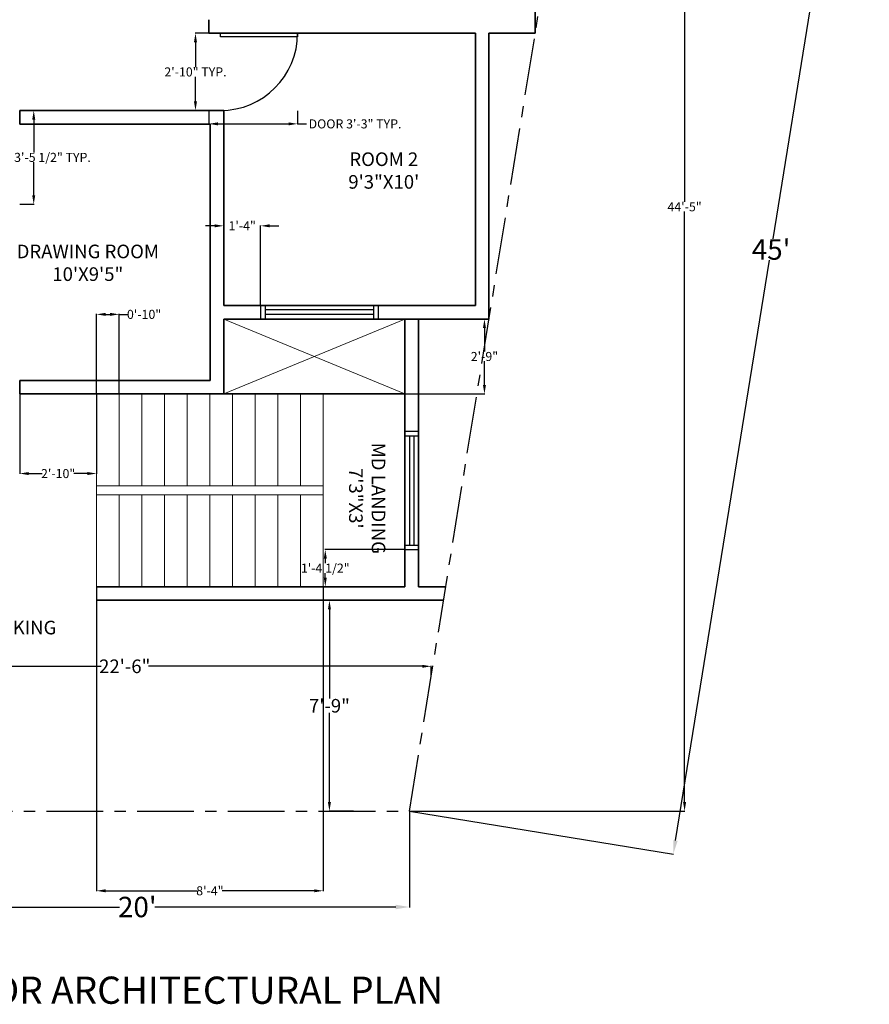
# Model space of a CAD drawing. Units: inches. Extents: x 1778 to 2384, y 384 to 1080.
# Tile 2 of 3: x 2009 to 2384, y 406 to 841. Entities that reach past the tile are written whole.
import ezdxf

# ---------------------------------------------------------------- set-up
doc = ezdxf.new("R2010")
doc.units = ezdxf.units.IN
doc.header["$MEASUREMENT"] = 0
doc.linetypes.add('CENTER', pattern=[2, 1.25, -0.25, 0.25, -0.25])
for name, color, linetype, lineweight in [('A-ANNO-DIMS', 2, 'Continuous', 18), ('A-ANNO-TEXT', 72, 'Continuous', 25), ('A-AREA-IDEN', 1, 'Continuous', 18), ('A-FLOR-STRS', 7, 'Continuous', 18), ('A-GLAZ', 4, 'Continuous', 18), ('A-WALL', 7, 'Continuous', 35), ('C-PROP', 13, 'CENTER', 25), ('DOOR', 13, 'Continuous', 25)]:
    doc.layers.add(name, color=color, linetype=linetype, lineweight=lineweight)
doc.styles.get("Standard").update_dxf_attribs({"font": 'arial.ttf'})
doc.dimstyles.get("Standard").update_dxf_attribs({"dimtxt": 4, "dimasz": 4, "dimexe": 0.18, "dimexo": 0.0625, "dimgap": 0.09, "dimtad": 0, "dimtih": 1, "dimtoh": 1, "dimdec": 0, "dimzin": 0, "dimdsep": 46, "dimlunit": 3, "dimtxsty": 'Standard', "dimcen": 0.09, "dimadec": 0, "dimazin": 0, "dimtfac": 1, "dimtdec": 0, "dimtofl": 0, "dimtmove": 0, "dimatfit": 3, "dimfxl": 1, "dimtolj": 1, "dimtzin": 0, "dimarcsym": 0})

# ---------------------------------------------------------------- blocks, each defined once
blk = doc.blocks.new('*D1')
at = {"layer": 'A-ANNO-DIMS', "color": 0, "lineweight": -2, "transparency": 16777216}
for p, q in [((2267.72, 1024.58), (2384.25, 1005.72)), ((2383.11, 999.82), (2341.67, 743.88)), ((2298.72, 478.61), (2340.16, 734.55)), ((2181.42, 491.52), (2297.94, 472.66))]:
    blk.add_line(p, q, dxfattribs=at)
at = {"layer": 'A-ANNO-DIMS', "color": 0, "transparency": 16777216}
for points in [[(2382.12, 999.98), (2384.1, 999.66), (2384.07, 1005.75)], [(2297.74, 478.77), (2299.71, 478.45), (2297.77, 472.69)]]:
    blk.add_solid(points, dxfattribs=at)
at = {"layer": 'Defpoints', "color": 0, "transparency": 16777216}
for p in [(2267.66, 1024.59), (2384.07, 1005.75), (2181.36, 491.53)]:
    blk.add_point(p, dxfattribs=at)
at = {"layer": 'A-ANNO-DIMS', "color": 0, "transparency": 16777216, "insert": (2340.92, 739.22), "char_height": 9, "attachment_point": 5}
blk.add_mtext("\\A1;45'", dxfattribs=at)
blk = doc.blocks.new('*D2')
at = {"layer": 'A-ANNO-DIMS', "color": 0, "lineweight": -2, "transparency": 16777216}
for p, q in [((1941.36, 491.47), (1941.36, 449.11)), ((2181.36, 491.47), (2181.36, 449.11)), ((1947.36, 449.29), (2053.55, 449.29)), ((2175.36, 449.29), (2069.16, 449.29))]:
    blk.add_line(p, q, dxfattribs=at)
at = {"layer": 'A-ANNO-DIMS', "color": 0, "transparency": 16777216}
for points in [[(1947.36, 450.29), (1947.36, 448.29), (1941.36, 449.29)], [(2175.36, 450.29), (2175.36, 448.29), (2181.36, 449.29)]]:
    blk.add_solid(points, dxfattribs=at)
at = {"layer": 'Defpoints', "color": 0, "transparency": 16777216}
for p in [(1941.36, 491.53), (2181.36, 491.53), (2181.36, 449.29)]:
    blk.add_point(p, dxfattribs=at)
at = {"layer": 'A-ANNO-DIMS', "color": 0, "transparency": 16777216, "insert": (2061.36, 449.29), "char_height": 9, "attachment_point": 5}
blk.add_mtext("\\A1;20'", dxfattribs=at)
blk = doc.blocks.new('*D4')
at = {"layer": 'A-ANNO-DIMS', "color": 0, "lineweight": -2, "transparency": 16777216}
for p, q in [((2238.23, 1077.18), (2031.58, 987.25)), ((2267.63, 1024.65), (2243.66, 1079.74)), ((1809.1, 890.44), (2015.76, 980.36)), ((1827.5, 833.12), (1803.53, 888.21))]:
    blk.add_line(p, q, dxfattribs=at)
at = {"layer": 'A-ANNO-DIMS', "color": 0, "transparency": 16777216}
for points in [[(2237.83, 1078.09), (2238.63, 1076.26), (2243.73, 1079.57)], [(1808.7, 891.35), (1809.5, 889.52), (1803.6, 888.04)]]:
    blk.add_solid(points, dxfattribs=at)
at = {"layer": 'Defpoints', "color": 0, "transparency": 16777216}
for p in [(2243.73, 1079.57), (2267.66, 1024.59), (1827.53, 833.06)]:
    blk.add_point(p, dxfattribs=at)
at = {"layer": 'A-ANNO-DIMS', "color": 0, "transparency": 16777216, "insert": (2023.67, 983.81), "char_height": 9, "attachment_point": 5}
blk.add_mtext("\\A1;40'", dxfattribs=at)
blk = doc.blocks.new('*D9')
at = {"layer": 'A-ANNO-DIMS', "color": 0, "lineweight": -2, "transparency": 16777216}
for p, q in [((1920.61, 553.84), (1920.61, 555.61)), ((1924.61, 555.43), (2045.38, 555.43)), ((2187.04, 555.43), (2066.27, 555.43)), ((2191.04, 551.41), (2191.04, 555.61))]:
    blk.add_line(p, q, dxfattribs=at)
at = {"layer": 'A-ANNO-DIMS', "color": 0, "transparency": 16777216}
for points in [[(1924.61, 556.1), (1924.61, 554.77), (1920.61, 555.43)], [(2187.04, 556.1), (2187.04, 554.77), (2191.04, 555.43)]]:
    blk.add_solid(points, dxfattribs=at)
at = {"layer": 'Defpoints', "color": 0, "transparency": 16777216}
for p in [(1920.61, 555.43), (1920.61, 553.77), (2191.04, 551.35)]:
    blk.add_point(p, dxfattribs=at)
at = {"layer": 'A-ANNO-DIMS', "color": 0, "transparency": 16777216, "insert": (2055.83, 555.43), "char_height": 6, "attachment_point": 5}
blk.add_mtext('\\A1;22\'-6"', dxfattribs=at)
blk = doc.blocks.new('*D12')
at = {"layer": 'A-ANNO-DIMS', "color": 0, "lineweight": -2, "transparency": 16777216}
for p, q in [((2156.73, 584.53), (2145.93, 584.53)), ((2146.11, 580.53), (2146.11, 541.19)), ((2146.11, 495.53), (2146.11, 534.88)), ((2156.73, 491.53), (2145.93, 491.53))]:
    blk.add_line(p, q, dxfattribs=at)
at = {"layer": 'A-ANNO-DIMS', "color": 0, "transparency": 16777216}
for points in [[(2145.44, 580.53), (2146.77, 580.53), (2146.11, 584.53)], [(2145.44, 495.53), (2146.77, 495.53), (2146.11, 491.53)]]:
    blk.add_solid(points, dxfattribs=at)
at = {"layer": 'Defpoints', "color": 0, "transparency": 16777216}
for p in [(2146.11, 584.53), (2156.8, 584.53), (2156.8, 491.53)]:
    blk.add_point(p, dxfattribs=at)
at = {"layer": 'A-ANNO-DIMS', "color": 0, "transparency": 16777216, "insert": (2146.11, 538.03), "char_height": 6, "attachment_point": 5}
blk.add_mtext('\\A1;7\'-9"', dxfattribs=at)
blk = doc.blocks.new('*U14')
for p, q in [((0, 0), (0, -6)), ((40, 0), (40, -6))]:
    blk.add_line(p, q)
blk.add_lwpolyline([(0, 0), (0, 40), (1.75, 40), (1.75, 0)], close=True)
blk.add_arc((0, 0), 40, 0, 90)
blk = doc.blocks.new('DOOR')
blk.add_blockref('*U14', (1810.9, 983.44))
blk = doc.blocks.new('WINDOW')
for p, q in [((1664.47, 998.33), (1658.47, 998.33)), ((1658.47, 950.33), (1664.47, 950.33))]:
    blk.add_line(p, q)
at = {"layer": 'DOOR'}
for p, q in [((1664.47, 1000.33), (1658.47, 1000.33)), ((1660.47, 998.33), (1660.47, 950.33)), ((1662.47, 998.33), (1662.47, 950.33)), ((1658.47, 948.33), (1664.47, 948.33))]:
    blk.add_line(p, q, dxfattribs=at)
blk = doc.blocks.new('WIN')
at = {"layer": 'Defpoints'}
for p, q in [((1658.47, 1000.33), (1658.47, 948.33)), ((1664.47, 1000.33), (1664.47, 948.33))]:
    blk.add_line(p, q, dxfattribs=at)
at = {"layer": 'DOOR'}
blk.add_blockref('WINDOW', (0, 0), dxfattribs=at)
blk = doc.blocks.new('*D21')
at = {"layer": 'A-ANNO-DIMS', "color": 0, "lineweight": -2, "transparency": 16777216}
for p, q in [((2009.54, 800.53), (2015.86, 800.53)), ((2015.68, 796.53), (2015.68, 782.01)), ((2015.68, 763.16), (2015.68, 777.68)), ((2009.54, 759.16), (2015.86, 759.16))]:
    blk.add_line(p, q, dxfattribs=at)
at = {"layer": 'A-ANNO-DIMS', "color": 0, "transparency": 16777216}
for points in [[(2015.01, 796.53), (2016.35, 796.53), (2015.68, 800.53)], [(2015.01, 763.16), (2016.35, 763.16), (2015.68, 759.16)]]:
    blk.add_solid(points, dxfattribs=at)
at = {"layer": 'Defpoints', "color": 0, "transparency": 16777216}
for p in [(2009.47, 800.53), (2009.47, 759.16), (2015.68, 759.16)]:
    blk.add_point(p, dxfattribs=at)
at = {"layer": 'A-ANNO-DIMS', "color": 0, "transparency": 16777216, "insert": (2015.68, 779.85), "char_height": 4, "attachment_point": 5}
blk.add_mtext('\\A1;DOOR 3\'-5 1/2" TYP.', dxfattribs=at)
blk = doc.blocks.new('*D23')
at = {"layer": 'A-ANNO-DIMS', "color": 0, "lineweight": -2, "transparency": 16777216}
for p, q in [((2092.89, 800.45), (2092.89, 794.45)), ((2132.06, 800.45), (2132.06, 794.45)), ((2096.89, 794.63), (2128.06, 794.63)), ((2132.06, 794.63), (2136.06, 794.63))]:
    blk.add_line(p, q, dxfattribs=at)
at = {"layer": 'A-ANNO-DIMS', "color": 0, "transparency": 16777216}
for points in [[(2096.89, 795.3), (2096.89, 793.97), (2092.89, 794.63)], [(2128.06, 795.3), (2128.06, 793.97), (2132.06, 794.63)]]:
    blk.add_solid(points, dxfattribs=at)
at = {"layer": 'Defpoints', "color": 0, "transparency": 16777216}
for p in [(2092.89, 800.51), (2132.06, 800.51), (2132.06, 794.63)]:
    blk.add_point(p, dxfattribs=at)
at = {"layer": 'A-ANNO-DIMS', "color": 0, "transparency": 16777216, "insert": (2157.4, 794.63), "char_height": 4, "attachment_point": 5}
blk.add_mtext('\\A1;DOOR 3\'-3" TYP.', dxfattribs=at)
blk = doc.blocks.new('*D24')
at = {"layer": 'A-ANNO-DIMS', "color": 0, "lineweight": -2, "transparency": 16777216}
for p, q in [((2092.83, 834.57), (2086.84, 834.57)), ((2087.02, 830.57), (2087.02, 819.67)), ((2087.02, 804.51), (2087.02, 815.41)), ((2092.83, 800.51), (2086.84, 800.51))]:
    blk.add_line(p, q, dxfattribs=at)
at = {"layer": 'A-ANNO-DIMS', "color": 0, "transparency": 16777216}
for points in [[(2086.35, 830.57), (2087.69, 830.57), (2087.02, 834.57)], [(2086.35, 804.51), (2087.69, 804.51), (2087.02, 800.51)]]:
    blk.add_solid(points, dxfattribs=at)
at = {"layer": 'Defpoints', "color": 0, "transparency": 16777216}
for p in [(2092.89, 834.57), (2087.02, 800.51), (2092.89, 800.51)]:
    blk.add_point(p, dxfattribs=at)
at = {"layer": 'A-ANNO-DIMS', "color": 0, "transparency": 16777216, "insert": (2087.02, 817.54), "char_height": 4, "attachment_point": 5}
blk.add_mtext('\\A1;2\'-10" TYP.', dxfattribs=at)
blk = doc.blocks.new('*D35')
at = {"layer": 'A-ANNO-DIMS', "color": 0, "lineweight": -2, "transparency": 16777216}
for p, q in [((2267.72, 1024.59), (2302.94, 1024.59)), ((2302.76, 1020.59), (2302.76, 760.19)), ((2302.76, 495.53), (2302.76, 755.94)), ((2181.42, 491.53), (2302.94, 491.53))]:
    blk.add_line(p, q, dxfattribs=at)
at = {"layer": 'A-ANNO-DIMS', "color": 0, "transparency": 16777216}
for points in [[(2302.09, 1020.59), (2303.43, 1020.59), (2302.76, 1024.59)], [(2302.09, 495.53), (2303.43, 495.53), (2302.76, 491.53)]]:
    blk.add_solid(points, dxfattribs=at)
at = {"layer": 'Defpoints', "color": 0, "transparency": 16777216}
for p in [(2267.66, 1024.59), (2302.76, 1024.59), (2181.36, 491.53)]:
    blk.add_point(p, dxfattribs=at)
at = {"layer": 'A-ANNO-DIMS', "color": 0, "transparency": 16777216, "insert": (2302.76, 758.06), "char_height": 4, "attachment_point": 5}
blk.add_mtext('\\A1;44\'-5"', dxfattribs=at)
blk = doc.blocks.new('*D36')
at = {"layer": 'A-ANNO-DIMS', "color": 0, "lineweight": -2, "transparency": 16777216}
for p, q in [((1827.53, 833.13), (1827.53, 1059.87)), ((1831.53, 1059.69), (2040.63, 1059.69)), ((2263.66, 1059.69), (2054.55, 1059.69)), ((2267.66, 1024.66), (2267.66, 1059.87))]:
    blk.add_line(p, q, dxfattribs=at)
at = {"layer": 'A-ANNO-DIMS', "color": 0, "transparency": 16777216}
for points in [[(1831.53, 1060.36), (1831.53, 1059.03), (1827.53, 1059.69)], [(2263.66, 1060.36), (2263.66, 1059.03), (2267.66, 1059.69)]]:
    blk.add_solid(points, dxfattribs=at)
at = {"layer": 'Defpoints', "color": 0, "transparency": 16777216}
for p in [(2267.66, 1059.69), (2267.66, 1024.59), (1827.53, 833.06)]:
    blk.add_point(p, dxfattribs=at)
at = {"layer": 'A-ANNO-DIMS', "color": 0, "transparency": 16777216, "insert": (2047.59, 1059.69), "char_height": 4, "attachment_point": 5}
blk.add_mtext('\\A1;36\'-8"', dxfattribs=at)
blk = doc.blocks.new('*D37')
at = {"layer": 'A-ANNO-DIMS', "color": 0, "lineweight": -2, "transparency": 16777216}
for p, q in [((2043.38, 590.47), (2043.38, 456.25)), ((2143.38, 590.47), (2143.38, 456.25)), ((2047.38, 456.43), (2087.98, 456.43)), ((2139.38, 456.43), (2098.79, 456.43))]:
    blk.add_line(p, q, dxfattribs=at)
at = {"layer": 'A-ANNO-DIMS', "color": 0, "transparency": 16777216}
for points in [[(2047.38, 457.1), (2047.38, 455.77), (2043.38, 456.43)], [(2139.38, 457.1), (2139.38, 455.77), (2143.38, 456.43)]]:
    blk.add_solid(points, dxfattribs=at)
at = {"layer": 'Defpoints', "color": 0, "transparency": 16777216}
for p in [(2043.38, 590.53), (2143.38, 590.53), (2143.38, 456.43)]:
    blk.add_point(p, dxfattribs=at)
at = {"layer": 'A-ANNO-DIMS', "color": 0, "transparency": 16777216, "insert": (2093.38, 456.43), "char_height": 4, "attachment_point": 5}
blk.add_mtext('\\A1;8\'-4"', dxfattribs=at)
blk = doc.blocks.new('*D38')
at = {"layer": 'A-ANNO-DIMS', "color": 0, "lineweight": -2, "transparency": 16777216}
for p, q in [((2043.38, 675.6), (2043.38, 710.81)), ((2047.38, 710.63), (2049.38, 710.63)), ((2053.38, 675.6), (2053.38, 710.81)), ((2053.38, 710.63), (2057.38, 710.63))]:
    blk.add_line(p, q, dxfattribs=at)
at = {"layer": 'A-ANNO-DIMS', "color": 0, "transparency": 16777216}
for points in [[(2047.38, 711.3), (2047.38, 709.97), (2043.38, 710.63)], [(2049.38, 711.3), (2049.38, 709.97), (2053.38, 710.63)]]:
    blk.add_solid(points, dxfattribs=at)
at = {"layer": 'Defpoints', "color": 0, "transparency": 16777216}
for p in [(2053.38, 710.63), (2043.38, 675.53), (2053.38, 675.53)]:
    blk.add_point(p, dxfattribs=at)
at = {"layer": 'A-ANNO-DIMS', "color": 0, "transparency": 16777216, "insert": (2064.35, 710.63), "char_height": 4, "attachment_point": 5}
blk.add_mtext('\\A1;0\'-10"', dxfattribs=at)
blk = doc.blocks.new('*D39')
at = {"layer": 'A-ANNO-DIMS', "color": 0, "lineweight": -2, "transparency": 16777216}
for p, q in [((2095.49, 749.67), (2091.49, 749.67)), ((2099.49, 714.63), (2099.49, 749.85)), ((2115.74, 714.63), (2115.74, 749.85)), ((2119.74, 749.67), (2123.74, 749.67))]:
    blk.add_line(p, q, dxfattribs=at)
at = {"layer": 'A-ANNO-DIMS', "color": 0, "transparency": 16777216}
for points in [[(2095.49, 750.34), (2095.49, 749), (2099.49, 749.67)], [(2119.74, 750.34), (2119.74, 749), (2115.74, 749.67)]]:
    blk.add_solid(points, dxfattribs=at)
at = {"layer": 'Defpoints', "color": 0, "transparency": 16777216}
for p in [(2115.74, 749.67), (2099.49, 714.57), (2115.74, 714.57)]:
    blk.add_point(p, dxfattribs=at)
at = {"layer": 'A-ANNO-DIMS', "color": 0, "transparency": 16777216, "insert": (2107.62, 749.67), "char_height": 4, "attachment_point": 5}
blk.add_mtext('\\A1;1\'-4"', dxfattribs=at)
blk = doc.blocks.new('*D40')
at = {"layer": 'A-ANNO-DIMS', "color": 0, "lineweight": -2, "transparency": 16777216}
for p, q in [((2179.32, 606.91), (2144.1, 606.91)), ((2144.28, 602.91), (2144.28, 600.88)), ((2144.28, 594.53), (2144.28, 596.56)), ((2179.32, 590.53), (2144.1, 590.53))]:
    blk.add_line(p, q, dxfattribs=at)
at = {"layer": 'A-ANNO-DIMS', "color": 0, "transparency": 16777216}
for points in [[(2143.62, 602.91), (2144.95, 602.91), (2144.28, 606.91)], [(2143.62, 594.53), (2144.95, 594.53), (2144.28, 590.53)]]:
    blk.add_solid(points, dxfattribs=at)
at = {"layer": 'Defpoints', "color": 0, "transparency": 16777216}
for p in [(2144.28, 606.91), (2179.38, 606.91), (2179.38, 590.53)]:
    blk.add_point(p, dxfattribs=at)
at = {"layer": 'A-ANNO-DIMS', "color": 0, "transparency": 16777216, "insert": (2144.28, 598.72), "char_height": 4, "attachment_point": 5}
blk.add_mtext('\\A1;1\'-4 1/2"', dxfattribs=at)
blk = doc.blocks.new('*D47')
at = {"layer": 'A-ANNO-DIMS', "color": 0, "lineweight": -2, "transparency": 16777216}
for p, q in [((2009.49, 675.47), (2009.49, 640.25)), ((2043.38, 675.47), (2043.38, 640.25)), ((2013.49, 640.43), (2019.45, 640.43)), ((2039.38, 640.43), (2033.43, 640.43))]:
    blk.add_line(p, q, dxfattribs=at)
at = {"layer": 'A-ANNO-DIMS', "color": 0, "transparency": 16777216}
for points in [[(2013.49, 641.1), (2013.49, 639.77), (2009.49, 640.43)], [(2039.38, 641.1), (2039.38, 639.77), (2043.38, 640.43)]]:
    blk.add_solid(points, dxfattribs=at)
at = {"layer": 'Defpoints', "color": 0, "transparency": 16777216}
for p in [(2009.49, 675.53), (2043.38, 675.53), (2009.49, 640.43)]:
    blk.add_point(p, dxfattribs=at)
at = {"layer": 'A-ANNO-DIMS', "color": 0, "transparency": 16777216, "insert": (2026.44, 640.43), "char_height": 4, "attachment_point": 5}
blk.add_mtext('\\A1;2\'-10"', dxfattribs=at)
blk = doc.blocks.new('*D48')
at = {"layer": 'A-ANNO-DIMS', "color": 0, "lineweight": -2, "transparency": 16777216}
for p, q in [((2179.45, 708.57), (2214.66, 708.57)), ((2214.48, 704.57), (2214.48, 694.18)), ((2214.48, 679.53), (2214.48, 689.92)), ((2179.45, 675.53), (2214.66, 675.53))]:
    blk.add_line(p, q, dxfattribs=at)
at = {"layer": 'A-ANNO-DIMS', "color": 0, "transparency": 16777216}
for points in [[(2213.82, 704.57), (2215.15, 704.57), (2214.48, 708.57)], [(2213.82, 679.53), (2215.15, 679.53), (2214.48, 675.53)]]:
    blk.add_solid(points, dxfattribs=at)
at = {"layer": 'Defpoints', "color": 0, "transparency": 16777216}
for p in [(2179.38, 708.57), (2179.38, 675.53), (2214.48, 675.53)]:
    blk.add_point(p, dxfattribs=at)
at = {"layer": 'A-ANNO-DIMS', "color": 0, "transparency": 16777216, "insert": (2214.48, 692.05), "char_height": 4, "attachment_point": 5}
blk.add_mtext('\\A1;2\'-9"', dxfattribs=at)

msp = doc.modelspace()

# ---------------------------------------------------------------- linework, layer by layer
at = {"layer": 'A-FLOR-STRS'}
for p, q in [((2099.49, 708.57), (2179.38, 675.53)), ((2179.38, 708.57), (2099.49, 675.53)), ((2043.38, 584.53), (2043.38, 675.53)), ((2053.38, 635.03), (2053.38, 675.53)), ((2063.38, 635.03), (2063.38, 675.53)), ((2073.38, 635.03), (2073.38, 675.53)), ((2083.38, 635.03), (2083.38, 675.53)), ((2093.38, 635.03), (2093.38, 675.53)), ((2103.38, 635.03), (2103.38, 675.53)), ((2113.38, 635.03), (2113.38, 675.53)), ((2123.38, 635.03), (2123.38, 675.53)), ((2133.38, 635.03), (2133.38, 675.53)), ((2143.38, 590.53), (2143.38, 675.53)), ((2143.38, 635.03), (2043.38, 635.03)), ((2143.38, 631.03), (2043.38, 631.03)), ((2053.38, 590.53), (2053.38, 631.03)), ((2063.38, 590.53), (2063.38, 631.03)), ((2073.38, 590.53), (2073.38, 631.03)), ((2083.38, 590.53), (2083.38, 631.03)), ((2093.38, 590.53), (2093.38, 631.03)), ((2103.38, 590.53), (2103.38, 631.03)), ((2113.38, 590.53), (2113.38, 631.03)), ((2123.38, 590.53), (2123.38, 631.03)), ((2133.38, 590.53), (2133.38, 631.03))]:
    msp.add_line(p, q, dxfattribs=at)
at = {"layer": 'A-WALL'}
for p, q in [((2236.89, 834.57), (2236.89, 942.57)), ((2092.89, 834.57), (2092.89, 840.57)), ((2099.49, 834.57), (2092.89, 834.57)), ((2210.49, 834.57), (2099.49, 834.57)), ((2210.49, 714.57), (2210.49, 834.57)), ((2236.89, 834.57), (2216.49, 834.57)), ((2216.49, 708.57), (2216.49, 834.57)), ((2009.49, 794.53), (2009.49, 800.53)), ((2099.49, 714.57), (2099.49, 800.53)), ((2093.49, 681.53), (2093.49, 794.53)), ((2210.49, 714.57), (2099.49, 714.57)), ((2216.49, 708.57), (2099.49, 708.57)), ((2099.49, 675.53), (2099.49, 708.57)), ((2179.38, 590.53), (2179.38, 708.57)), ((2185.38, 590.53), (2185.38, 708.57)), ((2009.49, 681.53), (2009.49, 675.53))]:
    msp.add_line(p, q, dxfattribs=at)
at = {"layer": 'A-WALL', "ltscale": 20}
for p, q in [((2009.49, 800.53), (2099.49, 800.53)), ((2009.49, 794.53), (2093.49, 794.53)), ((2009.49, 681.53), (2093.49, 681.53)), ((2009.49, 675.53), (2179.38, 675.53)), ((2043.38, 590.53), (2179.38, 590.53)), ((2185.38, 590.53), (2197.38, 590.53)), ((2043.38, 584.53), (2196.41, 584.53))]:
    msp.add_line(p, q, dxfattribs=at)
at = {"layer": 'C-PROP', "ltscale": 20}
for p, q in [((2181.36, 491.53), (2267.66, 1024.59)), ((1941.36, 491.53), (2181.36, 491.53))]:
    msp.add_line(p, q, dxfattribs=at)

# ---------------------------------------------------------------- block references
at = {"layer": 'A-GLAZ', "rotation": 270}
msp.add_blockref('WIN', (1167.41, 2373.04), dxfattribs=at)
at = {"layer": 'A-GLAZ'}
msp.add_blockref('WIN', (520.91, -341.42), dxfattribs=at)
at = {"layer": 'DOOR', "xscale": 0.851476605835392, "yscale": 0.851476605835392, "zscale": 0.851476605835392, "rotation": 270}
msp.add_blockref('DOOR', (1260.63, 2376.51), dxfattribs=at)

# ---------------------------------------------------------------- texts
at = {"layer": 'A-ANNO-TEXT', "insert": (1894.65, 418.6), "char_height": 12, "attachment_point": 1}
msp.add_mtext_dynamic_manual_height_columns('GROUND FLOOR ARCHITECTURAL PLAN', width=680.8928, gutter_width=1, heights=[0], dxfattribs=at)
at = {"layer": 'A-AREA-IDEN', "char_height": 6, "attachment_point": 2}
for s, insert in [('ROOM 2\\P9\'3"X10\'', (2170.09, 782.05)), ('DRAWING ROOM\\P10\'X9\'5"', (2039.54, 741.37)), ('PARKING', (2008.36, 575.52))]:
    msp.add_mtext_dynamic_manual_height_columns(s, width=72.6444, gutter_width=1, heights=[0], dxfattribs=dict(at, insert=insert))
at = {"layer": 'A-AREA-IDEN', "insert": (2170.77, 629.52), "char_height": 6, "attachment_point": 2, "rotation": 270}
msp.add_mtext_dynamic_manual_height_columns('MD LANDING\\P7\'3"X3\'', width=72.6444, gutter_width=1, heights=[0], dxfattribs=at)

# ---------------------------------------------------------------- dimensions: what is measured, and where the dimension line sits
at = {"layer": 'A-ANNO-DIMS'}
for p1, p2, distance, picture, middle in [((1827.53, 833.06), (2267.66, 1024.59), 59.96, '*D4', (2023.67, 983.81)), ((2181.36, 491.53), (2267.66, 1024.59), -117.92, '*D1', (2340.92, 739.22)), ((1941.36, 491.53), (2181.36, 491.53), -42.24, '*D2', (2061.36, 449.29))]:
    dim = msp.add_aligned_dim(p1=p1, p2=p2, distance=distance, dimstyle='Standard', override={"dimtxt": 9, "dimasz": 6, "dimclrd": 0, "dimclre": 0, "dimclrt": 0}, dxfattribs=at)
    dim.commit()
    dim.dimension.update_dxf_attribs({"geometry": picture, "text_midpoint": middle})
for base, p1, p2, override, picture, middle in [((2267.66, 1059.69), (1827.53, 833.06), (2267.66, 1024.59), {"dimdec": 1, "dimlfac": 1, "dimrnd": 0, "dimzin": 1, "dimdsep": 46, "dimlunit": 4, "dimfrac": 2}, '*D36', (2047.59, 1059.69)), ((2053.38, 710.63), (2043.38, 675.53), (2053.38, 675.53), {"dimdec": 1, "dimlfac": 1, "dimrnd": 0, "dimzin": 1, "dimdsep": 46, "dimlunit": 4, "dimfrac": 2}, '*D38', (2064.35, 710.63)), ((2143.38, 456.43), (2043.38, 590.53), (2143.38, 590.53), {"dimdec": 1, "dimlfac": 1, "dimrnd": 0, "dimzin": 1, "dimdsep": 46, "dimlunit": 4, "dimfrac": 2}, '*D37', (2093.38, 456.43)), ((1920.61, 555.43), (2191.04, 551.35), (1920.61, 553.77), {"dimtxt": 6, "dimclrd": 0, "dimclre": 0, "dimclrt": 0}, '*D9', (2055.83, 555.43))]:
    dim = msp.add_linear_dim(base=base, p1=p1, p2=p2, dimstyle='Standard', override=override, dxfattribs=at)
    dim.commit()
    dim.dimension.update_dxf_attribs({"geometry": picture, "text_midpoint": middle})
for base, p1, p2, angle, override, picture, middle in [((2302.76, 1024.59), (2181.36, 491.53), (2267.66, 1024.59), 90, {"dimdec": 1, "dimlfac": 1, "dimrnd": 0, "dimzin": 1, "dimdsep": 46, "dimlunit": 4, "dimfrac": 2}, '*D35', (2302.76, 758.06)), ((2115.7403, 749.6691), (2099.4945, 714.5691), (2115.7403, 714.5691), 0, {"dimdec": 1, "dimlfac": 1, "dimrnd": 0, "dimzin": 1, "dimdsep": 46, "dimlunit": 4, "dimfrac": 2}, '*D39', (2107.6174, 749.6691)), ((2214.48, 675.53), (2179.38, 708.57), (2179.38, 675.53), 270, {"dimdec": 1, "dimlfac": 1, "dimrnd": 0, "dimzin": 1, "dimdsep": 46, "dimlunit": 4, "dimfrac": 2}, '*D48', (2214.48, 692.05)), ((2009.49, 640.43), (2043.38, 675.53), (2009.49, 675.53), 180, {"dimdec": 1, "dimlfac": 1, "dimrnd": 0, "dimzin": 1, "dimdsep": 46, "dimlunit": 4, "dimfrac": 2}, '*D47', (2026.44, 640.43)), ((2144.28, 606.91), (2179.38, 590.53), (2179.38, 606.91), 90, {"dimdec": 1, "dimlfac": 1, "dimrnd": 0, "dimzin": 1, "dimdsep": 46, "dimlunit": 4, "dimfrac": 2}, '*D40', (2144.28, 598.72)), ((2146.11, 584.53), (2156.8, 491.53), (2156.8, 584.53), 90, {"dimtxt": 6, "dimclrd": 0, "dimclre": 0, "dimclrt": 0}, '*D12', (2146.11, 538.03))]:
    dim = msp.add_linear_dim(base=base, p1=p1, p2=p2, angle=angle, dimstyle='Standard', override=override, dxfattribs=at)
    dim.commit()
    dim.dimension.update_dxf_attribs({"geometry": picture, "text_midpoint": middle})
for base, p1, p2, text, picture, middle in [((2087.02, 800.51), (2092.89, 834.57), (2092.89, 800.51), '<> TYP.', '*D24', (2087.02, 817.54)), ((2015.68, 759.16), (2009.47, 800.53), (2009.47, 759.16), 'DOOR <> TYP.', '*D21', (2015.68, 779.85))]:
    dim = msp.add_linear_dim(base=base, p1=p1, p2=p2, angle=270, text=text, dimstyle='Standard', override={"dimdec": 1, "dimlfac": 1, "dimrnd": 0, "dimzin": 1, "dimdsep": 46, "dimlunit": 4, "dimfrac": 2}, dxfattribs=at)
    dim.commit()
    dim.dimension.update_dxf_attribs({"geometry": picture, "text_midpoint": middle})
dim = msp.add_linear_dim(base=(2132.06, 794.63), p1=(2092.89, 800.51), p2=(2132.06, 800.51), text='DOOR <> TYP.', dimstyle='Standard', override={"dimdec": 1, "dimlfac": 1, "dimrnd": 0, "dimzin": 1, "dimdsep": 46, "dimlunit": 4, "dimfrac": 2}, dxfattribs=at)
dim.commit()
dim.dimension.update_dxf_attribs({"geometry": '*D23', "text_midpoint": (2157.4, 794.63)})

doc.saveas('drawing.dxf')
